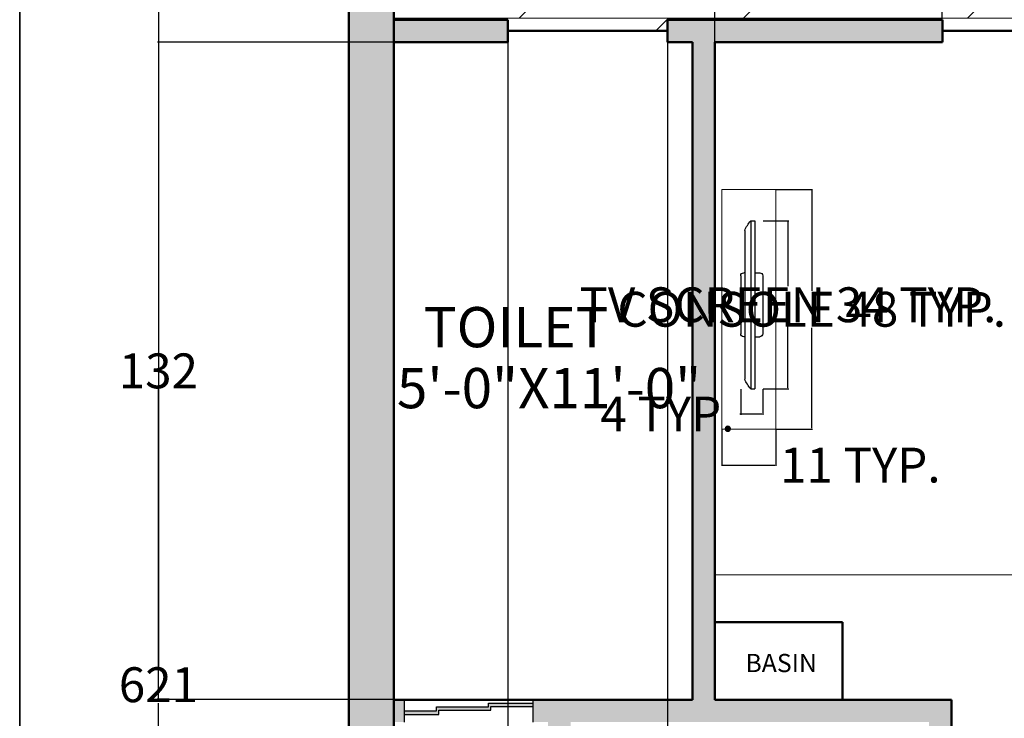
# Model space of a CAD drawing. Units: inches. Extents: x 1381 to 2246, y 1317 to 2168.
# Tile 5 of 15: x 1381 to 1579, y 1776 to 1916. Entities that reach past the tile are written whole.
import ezdxf

# ---------------------------------------------------------------- set-up
doc = ezdxf.new("R2010")
doc.units = ezdxf.units.IN
doc.header["$MEASUREMENT"] = 0
doc.layers.get('0').update_dxf_attribs({"color": 253})
for name, color, linetype, lineweight in [('A-ANNO-DIMS', 2, 'Continuous', 18), ('A-ANNO-TTLB', 7, 'Continuous', 35), ('A-AREA-IDEN', 3, 'Continuous', 25), ('A-FLOR-PATT', 252, 'Continuous', 13), ('A-FURN', 8, 'Continuous', 18), ('A-GLAZ', 4, 'Continuous', 25), ('A-WALL', 7, 'Continuous', 50)]:
    doc.layers.add(name, color=color, linetype=linetype, lineweight=lineweight)
doc.layers.add('furniture', color=250, linetype='Continuous')
doc.styles.get("Standard").update_dxf_attribs({"font": 'arial.ttf'})
doc.dimstyles.get("Standard").update_dxf_attribs({"dimtxt": 7, "dimasz": 0.18, "dimexe": 0.18, "dimexo": 0.0625, "dimgap": 0.09, "dimtad": 0, "dimtih": 1, "dimtoh": 1, "dimdec": 1, "dimzin": 0, "dimdsep": 46, "dimlunit": 3, "dimtxsty": 'Standard', "dimcen": 0.09, "dimadec": 0, "dimazin": 0, "dimtfac": 1, "dimtdec": 1, "dimtofl": 0, "dimtmove": 0, "dimatfit": 3, "dimfxl": 1, "dimtolj": 1, "dimtzin": 0, "dimarcsym": 0})

# ---------------------------------------------------------------- blocks, each defined once
blk = doc.blocks.new('PLASMA-LARGE')
at = {"layer": 'furniture'}
for p, q in [((-7.26, 0), (7.26, 0)), ((-18.61, -1), (18.61, -1)), ((-8, -1), (-8, -0.74)), ((8, -1), (8, -0.74)), ((-21, -2.5), (21, -2.5)), ((-21, -2.5), (-21, -3.5)), ((-21, -3.5), (21, -3.5)), ((-8, -3.5), (-8, -4.76)), ((8, -3.5), (8, -4.76)), ((21, -2.5), (21, -3.5)), ((-7.26, -5.5), (7.26, -5.5))]:
    blk.add_line(p, q, dxfattribs=at)
for centre, radius, start, end in [((-7.26, -0.74), 0.744, 90, 180), ((7.26, -0.74), 0.744, 0, 90), ((-13.97, -11.05), 11.07, 114.7602, 129.4175), ((13.97, -11.05), 11.07, 50.5825, 65.2398), ((-7.26, -4.76), 0.744, 180, 270), ((7.26, -4.76), 0.744, 270, 0)]:
    blk.add_arc(centre, radius, start, end, dxfattribs=at)
blk = doc.blocks.new('CONSOLE')
for p, q in [((10.82, 48.12), (0, 48.12)), ((0, 48.12), (0, 0)), ((10.82, 0), (10.82, 48.12)), ((0, 0), (10.82, 0))]:
    blk.add_line(p, q)
blk = doc.blocks.new('*D35')
at = {"layer": 'A-ANNO-DIMS', "color": 0, "lineweight": -2, "transparency": 16777216}
for p, q in [((1530.21, 1875.55), (1535.38, 1875.55)), ((1535.2, 1875.37), (1535.2, 1862.4)), ((1535.2, 1842), (1535.2, 1854.98)), ((1530.21, 1841.82), (1535.38, 1841.82))]:
    blk.add_line(p, q, dxfattribs=at)
at = {"layer": 'A-ANNO-DIMS', "color": 0, "transparency": 16777216}
for points in [[(1535.17, 1875.37), (1535.23, 1875.37), (1535.2, 1875.55)], [(1535.17, 1842), (1535.23, 1842), (1535.2, 1841.82)]]:
    blk.add_solid(points, dxfattribs=at)
at = {"layer": 'Defpoints', "color": 0, "transparency": 16777216}
for p in [(1530.14, 1875.55), (1530.14, 1841.82), (1535.2, 1841.82)]:
    blk.add_point(p, dxfattribs=at)
at = {"layer": 'A-ANNO-DIMS', "color": 0, "transparency": 16777216, "insert": (1535.2, 1858.69), "char_height": 7, "attachment_point": 5}
blk.add_mtext('\\A1;TV SCREEN 34 TYP.', dxfattribs=at)
blk = doc.blocks.new('*D36')
at = {"layer": 'A-ANNO-DIMS', "color": 0, "lineweight": -2, "transparency": 16777216}
for p, q in [((1525.73, 1841.76), (1525.73, 1836.58)), ((1530.14, 1841.76), (1530.14, 1836.58)), ((1525.73, 1836.76), (1525.55, 1836.76)), ((1529.96, 1836.76), (1525.91, 1836.76))]:
    blk.add_line(p, q, dxfattribs=at)
at = {"layer": 'A-ANNO-DIMS', "color": 0, "transparency": 16777216}
for points in [[(1525.91, 1836.79), (1525.91, 1836.73), (1525.73, 1836.76)], [(1529.96, 1836.79), (1529.96, 1836.73), (1530.14, 1836.76)]]:
    blk.add_solid(points, dxfattribs=at)
at = {"layer": 'Defpoints', "color": 0, "transparency": 16777216}
for p in [(1525.73, 1841.82), (1530.14, 1841.82), (1525.73, 1836.76)]:
    blk.add_point(p, dxfattribs=at)
at = {"layer": 'A-ANNO-DIMS', "color": 0, "transparency": 16777216, "insert": (1511, 1836.76), "char_height": 7, "attachment_point": 5}
blk.add_mtext('\\A1;4 TYP.', dxfattribs=at)
blk = doc.blocks.new('*D47')
at = {"layer": 'A-ANNO-DIMS', "color": 0, "lineweight": -2, "transparency": 16777216}
for p, q in [((1532.83, 1881.85), (1540.16, 1881.85)), ((1539.98, 1881.67), (1539.98, 1861.5)), ((1539.98, 1833.91), (1539.98, 1854.08)), ((1532.83, 1833.73), (1540.16, 1833.73))]:
    blk.add_line(p, q, dxfattribs=at)
at = {"layer": 'A-ANNO-DIMS', "color": 0, "transparency": 16777216}
for points in [[(1539.95, 1881.67), (1540.01, 1881.67), (1539.98, 1881.85)], [(1539.95, 1833.91), (1540.01, 1833.91), (1539.98, 1833.73)]]:
    blk.add_solid(points, dxfattribs=at)
at = {"layer": 'Defpoints', "color": 0, "transparency": 16777216}
for p in [(1532.76, 1881.85), (1539.98, 1881.85), (1532.76, 1833.73)]:
    blk.add_point(p, dxfattribs=at)
at = {"layer": 'A-ANNO-DIMS', "color": 0, "transparency": 16777216, "insert": (1539.98, 1857.79), "char_height": 7, "attachment_point": 5}
blk.add_mtext('\\A1;CONSOLE 48 TYP.', dxfattribs=at)
blk = doc.blocks.new('*D48')
at = {"layer": 'A-ANNO-DIMS', "color": 0, "lineweight": -2, "transparency": 16777216}
for p, q in [((1521.94, 1833.66), (1521.94, 1826.33)), ((1532.76, 1833.66), (1532.76, 1826.33)), ((1522.12, 1826.51), (1532.58, 1826.51)), ((1532.76, 1826.51), (1532.94, 1826.51))]:
    blk.add_line(p, q, dxfattribs=at)
at = {"layer": 'A-ANNO-DIMS', "color": 0, "transparency": 16777216}
for points in [[(1522.12, 1826.54), (1522.12, 1826.48), (1521.94, 1826.51)], [(1532.58, 1826.54), (1532.58, 1826.48), (1532.76, 1826.51)]]:
    blk.add_solid(points, dxfattribs=at)
at = {"layer": 'Defpoints', "color": 0, "transparency": 16777216}
for p in [(1521.94, 1833.73), (1532.76, 1833.73), (1532.76, 1826.51)]:
    blk.add_point(p, dxfattribs=at)
at = {"layer": 'A-ANNO-DIMS', "color": 0, "transparency": 16777216, "insert": (1549.74, 1826.51), "char_height": 7, "attachment_point": 5}
blk.add_mtext('\\A1;11 TYP.', dxfattribs=at)
blk = doc.blocks.new('*D50')
at = {"layer": 'A-ANNO-DIMS', "color": 0, "lineweight": -2, "transparency": 16777216}
for p, q in [((1446.99, 2092.92), (1408.62, 2092.92)), ((1408.8, 2092.74), (1408.8, 1786.08)), ((1408.8, 1472.1), (1408.8, 1778.75)), ((1446.99, 1471.92), (1408.62, 1471.92))]:
    blk.add_line(p, q, dxfattribs=at)
at = {"layer": 'A-ANNO-DIMS', "color": 0, "transparency": 16777216}
for points in [[(1408.77, 2092.74), (1408.83, 2092.74), (1408.8, 2092.92)], [(1408.77, 1472.1), (1408.83, 1472.1), (1408.8, 1471.92)]]:
    blk.add_solid(points, dxfattribs=at)
at = {"layer": 'Defpoints', "color": 0, "transparency": 16777216}
for p in [(1408.8, 2092.92), (1447.05, 2092.92), (1447.05, 1471.92)]:
    blk.add_point(p, dxfattribs=at)
at = {"layer": 'A-ANNO-DIMS', "color": 0, "transparency": 16777216, "insert": (1408.8, 1782.42), "char_height": 7, "attachment_point": 5}
blk.add_mtext('\\A1;621', dxfattribs=at)
blk = doc.blocks.new('*D56')
at = {"layer": 'A-ANNO-DIMS', "color": 0, "lineweight": -2, "transparency": 16777216}
for p, q in [((1455.99, 1911.42), (1408.62, 1911.42)), ((1408.8, 1911.24), (1408.8, 1849.08)), ((1408.8, 1779.6), (1408.8, 1841.75)), ((1455.99, 1779.42), (1408.62, 1779.42))]:
    blk.add_line(p, q, dxfattribs=at)
at = {"layer": 'A-ANNO-DIMS', "color": 0, "transparency": 16777216}
for points in [[(1408.77, 1911.24), (1408.83, 1911.24), (1408.8, 1911.42)], [(1408.77, 1779.6), (1408.83, 1779.6), (1408.8, 1779.42)]]:
    blk.add_solid(points, dxfattribs=at)
at = {"layer": 'Defpoints', "color": 0, "transparency": 16777216}
for p in [(1408.8, 1911.42), (1456.05, 1911.42), (1456.05, 1779.42)]:
    blk.add_point(p, dxfattribs=at)
at = {"layer": 'A-ANNO-DIMS', "color": 0, "transparency": 16777216, "insert": (1408.8, 1845.42), "char_height": 7, "attachment_point": 5}
blk.add_mtext('\\A1;132', dxfattribs=at)
blk = doc.blocks.new('*D67')
at = {"layer": 'A-ANNO-DIMS', "color": 0, "lineweight": -2, "transparency": 16777216}
for p, q in [((1456.050973, 1911.353813), (1456.050973, 1384.360695)), ((1478.962127, 1911.353813), (1478.962127, 1384.360695)), ((1455.870973, 1384.540695), (1455.690973, 1384.540695)), ((1479.142127, 1384.540695), (1479.322127, 1384.540695))]:
    blk.add_line(p, q, dxfattribs=at)
at = {"layer": 'A-ANNO-DIMS', "color": 0, "transparency": 16777216}
for points in [[(1455.870973, 1384.570695), (1455.870973, 1384.510695), (1456.050973, 1384.540695)], [(1479.142127, 1384.570695), (1479.142127, 1384.510695), (1478.962127, 1384.540695)]]:
    blk.add_solid(points, dxfattribs=at)
at = {"layer": 'Defpoints', "color": 0, "transparency": 16777216}
for p in [(1456.050973, 1911.416313), (1478.962127, 1911.416313), (1478.962127, 1384.540695)]:
    blk.add_point(p, dxfattribs=at)
at = {"layer": 'A-ANNO-DIMS', "color": 0, "transparency": 16777216, "insert": (1467.50655, 1384.540695), "char_height": 7, "attachment_point": 5}
blk.add_mtext('\\A1;22.91', dxfattribs=at)
blk = doc.blocks.new('*D68')
at = {"layer": 'A-ANNO-DIMS', "color": 0, "lineweight": -2, "transparency": 16777216}
for p, q in [((1478.96, 1911.35), (1478.96, 1384.36)), ((1511.02, 1911.35), (1511.02, 1384.36)), ((1479.14, 1384.54), (1480.39, 1384.54)), ((1510.84, 1384.54), (1509.59, 1384.54))]:
    blk.add_line(p, q, dxfattribs=at)
at = {"layer": 'A-ANNO-DIMS', "color": 0, "transparency": 16777216}
for points in [[(1479.14, 1384.57), (1479.14, 1384.51), (1478.96, 1384.54)], [(1510.84, 1384.57), (1510.84, 1384.51), (1511.02, 1384.54)]]:
    blk.add_solid(points, dxfattribs=at)
at = {"layer": 'Defpoints', "color": 0, "transparency": 16777216}
for p in [(1478.96, 1911.42), (1511.02, 1911.42), (1511.02, 1384.54)]:
    blk.add_point(p, dxfattribs=at)
at = {"layer": 'A-ANNO-DIMS', "color": 0, "transparency": 16777216, "insert": (1494.99, 1384.54), "char_height": 7, "attachment_point": 5}
blk.add_mtext('\\A1;32.054', dxfattribs=at)
blk = doc.blocks.new('*D71')
at = {"layer": 'A-ANNO-DIMS', "color": 0, "lineweight": -2, "transparency": 16777216}
for p, q in [((1520.55, 1911.48), (1520.55, 2160.41)), ((1520.73, 2160.23), (1531.34, 2160.23)), ((1566.03, 2160.23), (1555.42, 2160.23)), ((1566.21, 1911.48), (1566.21, 2160.41))]:
    blk.add_line(p, q, dxfattribs=at)
at = {"layer": 'A-ANNO-DIMS', "color": 0, "transparency": 16777216}
for points in [[(1520.73, 2160.26), (1520.73, 2160.2), (1520.55, 2160.23)], [(1566.03, 2160.26), (1566.03, 2160.2), (1566.21, 2160.23)]]:
    blk.add_solid(points, dxfattribs=at)
at = {"layer": 'Defpoints', "color": 0, "transparency": 16777216}
for p in [(1566.21, 2160.23), (1520.55, 1911.42), (1566.21, 1911.42)]:
    blk.add_point(p, dxfattribs=at)
at = {"layer": 'A-ANNO-DIMS', "color": 0, "transparency": 16777216, "insert": (1543.38, 2160.23), "char_height": 7, "attachment_point": 5}
blk.add_mtext('\\A1;45.66', dxfattribs=at)
blk = doc.blocks.new('*D72')
at = {"layer": 'A-ANNO-DIMS', "color": 0, "lineweight": -2, "transparency": 16777216}
for p, q in [((1566.21, 1911.48), (1566.21, 2160.41)), ((1566.39, 2160.23), (1573.94, 2160.23)), ((1611.06, 2160.23), (1603.51, 2160.23)), ((1611.24, 1911.48), (1611.24, 2160.41))]:
    blk.add_line(p, q, dxfattribs=at)
at = {"layer": 'A-ANNO-DIMS', "color": 0, "transparency": 16777216}
for points in [[(1566.39, 2160.26), (1566.39, 2160.2), (1566.21, 2160.23)], [(1611.06, 2160.26), (1611.06, 2160.2), (1611.24, 2160.23)]]:
    blk.add_solid(points, dxfattribs=at)
at = {"layer": 'Defpoints', "color": 0, "transparency": 16777216}
for p in [(1611.24, 2160.23), (1566.21, 1911.42), (1611.24, 1911.42)]:
    blk.add_point(p, dxfattribs=at)
at = {"layer": 'A-ANNO-DIMS', "color": 0, "transparency": 16777216, "insert": (1588.72, 2160.23), "char_height": 7, "attachment_point": 5}
blk.add_mtext('\\A1;45.025', dxfattribs=at)

msp = doc.modelspace()

# ---------------------------------------------------------------- hatches: boundary and pattern name
at = {"layer": 'A-FLOR-PATT'}
h = msp.add_hatch(dxfattribs=at)
h.set_pattern_fill('DOLMIT', color=256, scale=15)
h.paths.add_polyline_path([(1618.051, 2040.2358), (1618.051, 2083.9163), (1517.1194, 2083.9163), (1517.1194, 2057.4148), (1456.051, 2057.4148), (1456.051, 1915.9163), (1478.9621, 1915.9163), (1478.9621, 1913.6663), (1511.016, 1913.6663), (1511.016, 1915.9163), (1566.2107, 1915.9163), (1566.2107, 1913.6663), (1611.2353, 1913.6663), (1611.2353, 1915.9163), (1618.051, 1915.9163)])
h.paths.add_polyline_path([(1526.2629, 2024.4608), (1526.2629, 1955.9789), (1497.7075, 1955.9789), (1497.7075, 1962.7697), (1471.5798, 1962.7697), (1471.6908, 1951.263), (1458.495, 1951.263), (1458.384, 1962.7697), (1458.384, 2014.1291), (1458.273, 2025.6358), (1471.4689, 2025.6358), (1471.5798, 2014.1291), (1497.7075, 2014.1291), (1497.7075, 2024.4608)], flags=16)
h.paths.add_polyline_path([(1475.9437, 2014.0737), (1475.9437, 2004.8072), (1469.1114, 2004.8072), (1469.0654, 2004.7449), (1469.0654, 1968.5691), (1461.3046, 1968.5691), (1461.3046, 1983.6181), (1469.0654, 1983.6181), (1469.0654, 1989.7582), (1461.3046, 1989.7582), (1461.3046, 2004.8072), (1469.1114, 2004.8072)], flags=0)
h.paths.add_polyline_path([(1469.1187, 2020.1923, -1), (1460.6232, 2020.1923, -1)], flags=0)
h.paths.add_polyline_path([(1469.2296, 1957.3262, -1), (1460.7342, 1957.3262, -1)], flags=0)
h.paths.add_polyline_path([(1533.5744, 1985.8776), (1602.6925, 1985.8776), (1602.6925, 1998.2538), (1533.5744, 1998.2538)], flags=24)
h.paths.add_polyline_path([(1535.349, 2002.3157), (1604.0842, 2002.3157), (1604.0842, 2014.8488), (1535.349, 2014.8488)], flags=24)
at = {"layer": 'A-GLAZ'}
h = msp.add_hatch(color=256, dxfattribs=at)
h.dxf.hatch_style = 1
h.paths.add_polyline_path([(1456.051, 2083.9163), (1737.551, 2083.9163), (1737.551, 1677.4163), (1732.8596, 1677.4163), (1732.8596, 1672.9163), (1737.551, 1672.9163), (1737.551, 1471.9163), (1746.551, 1471.9163), (1746.551, 2092.9163), (1447.051, 2092.9163), (1447.051, 2083.9163), (1447.051, 1471.9163), (1488.6632, 1471.9163), (1488.6632, 1480.9163), (1456.051, 1480.9163), (1456.051, 1710.4163), (1517.1194, 1710.4163), (1517.1194, 1714.9163), (1491.551, 1714.9163), (1491.551, 1729.193), (1487.051, 1729.193), (1487.051, 1714.9163), (1456.051, 1714.9163)])
h.paths.add_polyline_path([(1622.551, 2035.4163), (1625.0954, 2035.4163), (1625.0954, 2039.9163), (1618.051, 2039.9163), (1618.051, 1915.9163), (1611.2353, 1915.9163), (1611.2353, 1911.4163), (1626.5102, 1911.4163), (1626.5102, 1915.9163), (1622.551, 1915.9163)], flags=17)
h.paths.add_polyline_path([(1737.551, 1915.9163), (1668.5102, 1915.9163), (1668.5102, 1911.4163), (1737.551, 1911.4163)], flags=17)
h.paths.add_polyline_path([(1682.2831, 2039.9163), (1655.8191, 2039.9163), (1655.8191, 2035.4163), (1682.2831, 2035.4163)], flags=17)
h.paths.add_polyline_path([(1737.551, 2039.9163), (1725.9636, 2039.9163), (1725.9636, 2035.4163), (1737.551, 2035.4163)], flags=17)
h.paths.add_polyline_path([(1684.2508, 1711.4667), (1740.8192, 1711.4667), (1740.8192, 1723.8346), (1684.2508, 1723.8346)], flags=25)
h = msp.add_hatch(color=256, dxfattribs=at)
h.dxf.hatch_style = 1
h.paths.add_polyline_path([(1478.9621, 1915.9163), (1456.051, 1915.9163), (1456.051, 1911.4163), (1478.9621, 1911.4163)])
h.paths.add_polyline_path([(1566.2107, 1915.9163), (1511.016, 1915.9163), (1511.016, 1911.4163), (1516.051, 1911.4163), (1516.051, 1779.4163), (1484.0852, 1779.4163), (1484.0852, 1774.9163), (1487.051, 1774.9163), (1487.051, 1755.1129), (1491.551, 1755.1129), (1491.551, 1774.9163), (1563.551, 1774.9163), (1563.551, 1770.3401), (1568.051, 1770.3401), (1568.051, 1779.4163), (1520.551, 1779.4163), (1520.551, 1911.4163), (1566.2107, 1911.4163)])
h.paths.add_polyline_path([(1568.051, 1734.7997), (1563.551, 1734.7997), (1563.551, 1714.9163), (1557.5961, 1714.9163), (1557.5961, 1710.4163), (1568.051, 1710.4163)])
h.paths.add_polyline_path([(1458.1653, 1779.4163), (1456.051, 1779.4163), (1456.051, 1774.9163), (1458.1653, 1774.9163)])
h.paths.add_polyline_path([(1684.551, 1746.8536), (1680.051, 1746.8536), (1680.051, 1677.4163), (1673.5117, 1677.4163), (1673.5117, 1672.9163), (1699.1735, 1672.9163), (1699.1735, 1677.4163), (1684.551, 1677.4163)])
h.paths.add_polyline_path([(1613.551, 1746.8536), (1609.051, 1746.8536), (1609.051, 1624.2465), (1618.051, 1624.2465), (1618.051, 1672.9163), (1625.5117, 1672.9163), (1625.5117, 1677.4163), (1613.551, 1677.4163)])
h.paths.add_polyline_path([(1618.051, 1585.1257), (1609.051, 1585.1257), (1609.051, 1569.4163), (1618.051, 1569.4163)])
h.paths.add_polyline_path([(1545.7088, 1578.4163), (1456.051, 1578.4163), (1456.051, 1569.4163), (1545.7088, 1569.4163)])
h.paths.add_polyline_path([(1594.0453, 1480.9163), (1536.6467, 1480.9163), (1536.6467, 1471.9163), (1594.0453, 1471.9163)])
h = msp.add_hatch(color=256, dxfattribs=at)
h.dxf.hatch_style = 1
h.paths.add_polyline_path([(1465.1314, 1777.3422), (1475.5261, 1777.3422), (1475.5261, 1778.0682), (1484.0852, 1778.0682), (1484.0852, 1778.7283), (1475.0856, 1778.7283), (1475.0856, 1777.9582), (1464.6469, 1777.9582), (1464.6469, 1777.1663), (1458.1653, 1777.1663), (1458.1653, 1776.4401), (1465.1314, 1776.4401)])

# ---------------------------------------------------------------- linework, layer by layer
at = {"layer": 'A-ANNO-DIMS'}
msp.add_line((1520.551, 1804.4959), (1737.551, 1804.4959), dxfattribs=at)
at = {"layer": 'A-ANNO-TTLB'}
msp.add_line((1380.9518, 1316.7761), (1380.9518, 2167.8236), dxfattribs=at)
at = {"layer": 'A-GLAZ'}
for p, q in [((1458.1653, 1779.4163), (1458.1653, 1774.9163)), ((1484.0852, 1779.4163), (1458.1653, 1779.4163)), ((1484.0852, 1774.9163), (1484.0852, 1779.4163)), ((1464.6469, 1777.1663), (1464.6469, 1777.9582)), ((1464.6469, 1777.9582), (1475.0856, 1777.9582)), ((1475.0856, 1777.9582), (1475.0856, 1778.7283)), ((1475.0856, 1778.7283), (1484.0852, 1778.7283)), ((1475.5261, 1777.3422), (1475.5261, 1778.0682)), ((1475.5261, 1778.0682), (1484.0852, 1778.0682)), ((1458.1653, 1777.1663), (1464.6469, 1777.1663)), ((1458.1653, 1776.4401), (1458.1653, 1776.4401)), ((1458.1653, 1776.4401), (1465.1314, 1776.4401)), ((1465.1314, 1776.4401), (1465.1314, 1777.3422)), ((1465.1314, 1777.3422), (1475.5261, 1777.3422))]:
    msp.add_line(p, q, dxfattribs=at)
at = {"layer": 'A-WALL'}
for p, q in [((1447.051, 2083.9163), (1447.051, 1471.9163)), ((1456.051, 2083.9163), (1456.051, 1714.9163)), ((1456.051, 1915.9163), (1478.9621, 1915.9163)), ((1478.9621, 1915.9163), (1478.9621, 1911.4163)), ((1511.016, 1915.9163), (1511.016, 1911.4163)), ((1511.016, 1915.9163), (1566.2107, 1915.9163)), ((1566.2107, 1915.9163), (1566.2107, 1911.4163)), ((1478.9621, 1913.6663), (1511.016, 1913.6663)), ((1566.2107, 1913.6663), (1611.2353, 1913.6663)), ((1456.051, 1911.4163), (1478.9621, 1911.4163)), ((1511.016, 1911.4163), (1516.051, 1911.4163)), ((1516.051, 1911.4163), (1516.051, 1779.4163)), ((1520.551, 1911.4163), (1520.551, 1779.4163)), ((1520.551, 1911.4163), (1566.2107, 1911.4163)), ((1520.551, 1794.9885), (1520.551, 1794.9885)), ((1520.551, 1794.9885), (1546.1766, 1794.9885)), ((1546.1766, 1794.9885), (1546.1766, 1779.4163)), ((1456.051, 1779.4163), (1516.051, 1779.4163)), ((1520.551, 1779.4163), (1568.051, 1779.4163)), ((1568.051, 1779.4163), (1568.051, 1770.3401))]:
    msp.add_line(p, q, dxfattribs=at)

# ---------------------------------------------------------------- block references
at = {"layer": 'A-FURN'}
msp.add_blockref('CONSOLE', (1521.942, 1833.726), dxfattribs=at)
at = {"layer": 'A-FURN', "xscale": -0.8031214548296134, "yscale": 0.8031214548296134, "zscale": 0.8031214548296134, "rotation": 90}
msp.add_blockref('PLASMA-LARGE', (1525.7255, 1858.6869), dxfattribs=at)

# ---------------------------------------------------------------- texts
at = {"layer": 'A-AREA-IDEN'}
for s, height, p in [('TOILET', 8.07451, (1462.0915, 1850.1635)), ('5\'-0"X11\'-0"', 8.074511, (1456.6976, 1837.9238)), ('BASIN', 3.66027, (1526.6661, 1784.9463))]:
    msp.add_text(s, height=height, dxfattribs=at).set_placement(p)

# ---------------------------------------------------------------- dimensions: what is measured, and where the dimension line sits
at = {"layer": 'A-ANNO-DIMS'}
for base, p1, p2, override, picture, middle in [((1566.2107, 2160.2332), (1520.551, 1911.4163), (1566.2107, 1911.4163), {"dimdec": 2, "dimlfac": 1, "dimrnd": 0, "dimzin": 0, "dimdsep": 46, "dimlunit": 2}, '*D71', (1543.3808, 2160.2332)), ((1611.2353, 2160.2332), (1566.2107, 1911.4163), (1611.2353, 1911.4163), {"dimdec": 3, "dimlfac": 1, "dimrnd": 0, "dimzin": 0, "dimdsep": 46, "dimlunit": 2}, '*D72', (1588.723, 2160.2332)), ((1478.9621, 1384.5407), (1456.051, 1911.4163), (1478.9621, 1911.4163), {"dimdec": 2, "dimlfac": 1, "dimrnd": 0, "dimzin": 0, "dimdsep": 46, "dimlunit": 2}, '*D67', (1467.5066, 1384.5407)), ((1511.016, 1384.5407), (1478.9621, 1911.4163), (1511.016, 1911.4163), {"dimdec": 3, "dimlfac": 1, "dimrnd": 0, "dimzin": 0, "dimdsep": 46, "dimlunit": 2}, '*D68', (1494.9891, 1384.5407))]:
    dim = msp.add_linear_dim(base=base, p1=p1, p2=p2, dimstyle='Standard', override=override, dxfattribs=at)
    dim.commit()
    dim.dimension.update_dxf_attribs({"geometry": picture, "text_midpoint": middle})
for base, p1, p2, picture, middle in [((1408.801, 2092.9163), (1447.051, 1471.9163), (1447.051, 2092.9163), '*D50', (1408.801, 1782.4163)), ((1408.801, 1911.4163), (1456.051, 1779.4163), (1456.051, 1911.4163), '*D56', (1408.801, 1845.4163))]:
    dim = msp.add_linear_dim(base=base, p1=p1, p2=p2, angle=90, dimstyle='Standard', override={"dimdec": 0, "dimlfac": 1, "dimrnd": 0, "dimzin": 0, "dimdsep": 46, "dimlunit": 2}, dxfattribs=at)
    dim.commit()
    dim.dimension.update_dxf_attribs({"geometry": picture, "text_midpoint": middle})
for base, p1, p2, angle, text, picture, middle in [((1535.2023, 1841.8213), (1530.1427, 1875.5524), (1530.1427, 1841.8213), 270, 'TV SCREEN <> TYP.', '*D35', (1535.2023, 1858.6869)), ((1539.9834, 1881.8501), (1532.7647, 1833.7256), (1532.7647, 1881.8501), 90, 'CONSOLE <> TYP.', '*D47', (1539.9834, 1857.7879)), ((1525.7255, 1836.7617), (1530.1427, 1841.8213), (1525.7255, 1841.8213), 180, '<> TYP.', '*D36', (1510.9971, 1836.7617))]:
    dim = msp.add_linear_dim(base=base, p1=p1, p2=p2, angle=angle, text=text, dimstyle='Standard', override={"dimdec": 0, "dimrnd": 0, "dimzin": 0, "dimlunit": 2}, dxfattribs=at)
    dim.commit()
    dim.dimension.update_dxf_attribs({"geometry": picture, "text_midpoint": middle})
dim = msp.add_linear_dim(base=(1532.7647, 1826.5069), p1=(1521.9424, 1833.7256), p2=(1532.7647, 1833.7256), text='<> TYP.', dimstyle='Standard', override={"dimdec": 0, "dimrnd": 0, "dimzin": 0, "dimlunit": 2}, dxfattribs=at)
dim.commit()
dim.dimension.update_dxf_attribs({"geometry": '*D48', "text_midpoint": (1549.7421, 1826.5069)})

doc.saveas('drawing.dxf')
